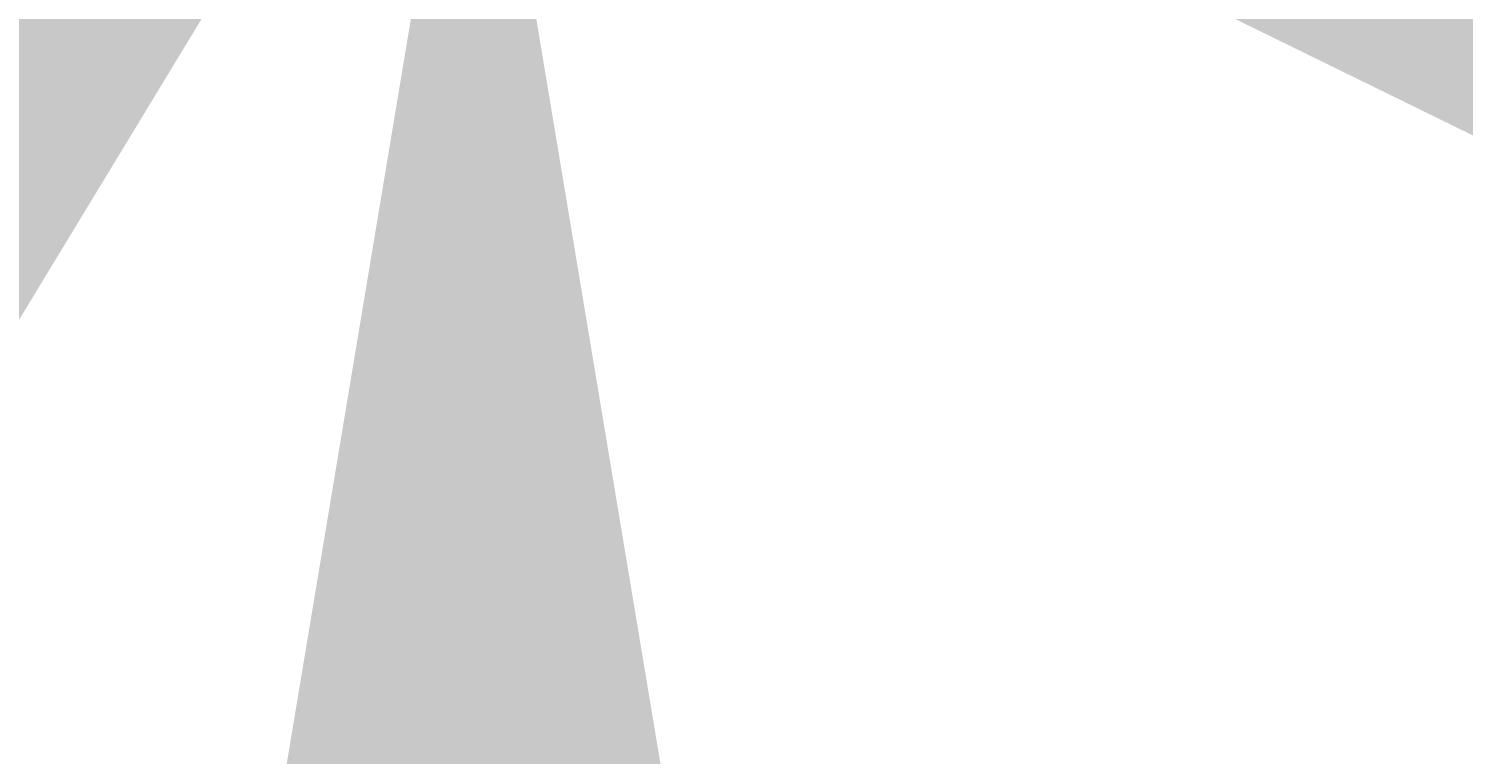
# Model space of a CAD drawing. Units: millimetres. Extents: x -22994 to 29398, y -19990 to 20176.
# Tile 3 of 135: x -2139 to 5745, y -5973 to -1986. Entities that reach past the tile are written whole.
import ezdxf

# ---------------------------------------------------------------- set-up
doc = ezdxf.new("R2010")
doc.units = ezdxf.units.MM
doc.header["$MEASUREMENT"] = 0
doc.layers.add('M-DIMS', color=2, linetype='Continuous', lineweight=18)
doc.styles.get("Standard").update_dxf_attribs({"font": 'arial.ttf'})
doc.dimstyles.get("Standard").update_dxf_attribs({"dimtxt": 0.18, "dimasz": 10000, "dimexe": 0.18, "dimexo": 0.0625, "dimgap": 0.09, "dimtad": 0, "dimtih": 1, "dimtoh": 1, "dimdec": 0, "dimzin": 0, "dimdsep": 46, "dimtxsty": 'Standard', "dimcen": 0.09, "dimadec": 0, "dimazin": 0, "dimtfac": 1, "dimtdec": 0, "dimtofl": 0, "dimtmove": 0, "dimatfit": 3, "dimfxl": 1, "dimtolj": 1, "dimtzin": 0, "dimlwd": 30, "dimarcsym": 0})

# ---------------------------------------------------------------- blocks, each defined once
blk = doc.blocks.new('*D9')
at = {"layer": 'Defpoints', "color": 0, "transparency": 16777216}
for p in [(187.3, 176.4), (306.2, 176.4), (290.9, 10.3)]:
    blk.add_point(p, dxfattribs=at)
at = {"layer": 'M-DIMS', "color": 0, "lineweight": 30, "transparency": 16777216}
for p, q in [((306.2, 10176.4), (306.2, 20176.4)), ((306.2, -9989.7), (306.2, -19989.7))]:
    blk.add_line(p, q, dxfattribs=at)
at = {"layer": 'M-DIMS', "color": 0, "lineweight": -2, "transparency": 16777216}
for p, q in [((187.3, 176.4), (306.4, 176.4)), ((290.9, 10.3), (306.4, 10.3))]:
    blk.add_line(p, q, dxfattribs=at)
at = {"layer": 'M-DIMS', "color": 0, "transparency": 16777216}
for points in [[(-1360.5, 10176.4), (1972.9, 10176.4), (306.2, 176.4)], [(-1360.5, -9989.7), (1972.9, -9989.7), (306.2, 10.3)]]:
    blk.add_solid(points, dxfattribs=at)
at = {"layer": 'M-DIMS', "color": 0, "transparency": 16777216, "insert": (306.2, 93.3), "char_height": 0.18, "attachment_point": 5}
blk.add_mtext('\\A1;166.1', dxfattribs=at)
blk = doc.blocks.new('*D15')
at = {"layer": 'Defpoints', "color": 0, "transparency": 16777216}
for p in [(173.3, 154.8), (173.3, 136.1), (306.2, 136.1)]:
    blk.add_point(p, dxfattribs=at)
at = {"layer": 'M-DIMS', "color": 0, "lineweight": 30, "transparency": 16777216}
for p, q in [((306.2, 10154.8), (306.2, 20154.8)), ((306.2, -9863.9), (306.2, -19863.9))]:
    blk.add_line(p, q, dxfattribs=at)
at = {"layer": 'M-DIMS', "color": 0, "lineweight": -2, "transparency": 16777216}
for p, q in [((173.4, 154.8), (306.4, 154.8)), ((173.4, 136.1), (306.4, 136.1))]:
    blk.add_line(p, q, dxfattribs=at)
at = {"layer": 'M-DIMS', "color": 0, "transparency": 16777216}
for points in [[(-1360.5, 10154.8), (1972.9, 10154.8), (306.2, 154.8)], [(-1360.5, -9863.9), (1972.9, -9863.9), (306.2, 136.1)]]:
    blk.add_solid(points, dxfattribs=at)
at = {"layer": 'M-DIMS', "color": 0, "transparency": 16777216, "insert": (306.2, 145.4), "char_height": 0.18, "attachment_point": 5}
blk.add_mtext('\\A1;18.717', dxfattribs=at)
blk = doc.blocks.new('*D28')
at = {"layer": 'Defpoints', "color": 0, "transparency": 16777216}
for p in [(188.1, 48), (188.1, 31), (306.2, 48)]:
    blk.add_point(p, dxfattribs=at)
at = {"layer": 'M-DIMS', "color": 0, "lineweight": 30, "transparency": 16777216}
for p, q in [((306.2, 10048), (306.2, 20048)), ((306.2, -9969), (306.2, -19969))]:
    blk.add_line(p, q, dxfattribs=at)
at = {"layer": 'M-DIMS', "color": 0, "lineweight": -2, "transparency": 16777216}
for p, q in [((188.2, 48), (306.4, 48)), ((188.2, 31), (306.4, 31))]:
    blk.add_line(p, q, dxfattribs=at)
at = {"layer": 'M-DIMS', "color": 0, "transparency": 16777216}
for points in [[(-1360.5, 10048), (1972.9, 10048), (306.2, 48)], [(-1360.5, -9969), (1972.9, -9969), (306.2, 31)]]:
    blk.add_solid(points, dxfattribs=at)
at = {"layer": 'M-DIMS', "color": 0, "transparency": 16777216, "insert": (306.2, 39.5), "char_height": 0.18, "attachment_point": 5}
blk.add_mtext('\\A1;17.045', dxfattribs=at)
blk = doc.blocks.new('*D32')
at = {"layer": 'Defpoints', "color": 0, "transparency": 16777216}
for p in [(52.4, 113.1), (57.2, 118.6)]:
    blk.add_point(p, dxfattribs=at)
at = {"layer": 'M-DIMS', "color": 0, "lineweight": -2, "transparency": 16777216}
for p, q in [((57.1, 118.6), (57.3, 118.6)), ((57.2, 118.5), (57.2, 118.7))]:
    blk.add_line(p, q, dxfattribs=at)
at = {"layer": 'M-DIMS', "color": 0, "lineweight": 30, "transparency": 16777216}
for p, q in [((-12992.5, -15047), (-6470.1, -7467)), ((-22992.5, -15047), (-12992.5, -15047))]:
    blk.add_line(p, q, dxfattribs=at)
at = {"layer": 'M-DIMS', "color": 0, "transparency": 16777216}
blk.add_solid([(-7733.4, -6379.9), (-5206.7, -8554), (52.4, 113.1)], dxfattribs=at)
at = {"layer": 'M-DIMS', "color": 0, "transparency": 16777216, "insert": (-22993.2, -15047), "char_height": 0.18, "attachment_point": 5}
blk.add_mtext('\\A1;2X R7.284', dxfattribs=at)
blk = doc.blocks.new('*D33')
at = {"layer": 'Defpoints', "color": 0, "transparency": 16777216}
for p in [(229.6, 154.4), (233, 153.4)]:
    blk.add_point(p, dxfattribs=at)
at = {"layer": 'M-DIMS', "color": 0, "lineweight": -2, "transparency": 16777216}
for p, q in [((229.5, 154.4), (229.7, 154.4)), ((229.6, 154.3), (229.6, 154.5))]:
    blk.add_line(p, q, dxfattribs=at)
at = {"layer": 'M-DIMS', "color": 0, "lineweight": 30, "transparency": 16777216}
for p, q in [((19396.3, -5570.8), (9814.7, -2708.7)), ((29396.3, -5570.8), (19396.3, -5570.8))]:
    blk.add_line(p, q, dxfattribs=at)
at = {"layer": 'M-DIMS', "color": 0, "transparency": 16777216}
blk.add_solid([(10291.7, -1111.8), (9337.7, -4305.7), (233, 153.4)], dxfattribs=at)
at = {"layer": 'M-DIMS', "color": 0, "transparency": 16777216, "insert": (29397, -5570.8), "char_height": 0.18, "attachment_point": 5}
blk.add_mtext('\\A1;6X R3.586', dxfattribs=at)

msp = doc.modelspace()

# ---------------------------------------------------------------- dimensions: what is measured, and where the dimension line sits
at = {"layer": 'M-DIMS'}
for base, p1, p2, override, picture, middle in [((306.202, 176.3662), (290.852, 10.2713), (187.2647, 176.3662), {"dimdec": 1, "dimlfac": 1, "dimrnd": 0, "dimzin": 0, "dimdsep": 46, "dimlunit": 2}, '*D9', (306.202, 93.3187)), ((306.202, 136.0713), (173.3459, 154.788), (173.3459, 136.0713), {"dimdec": 3, "dimlfac": 1, "dimrnd": 0, "dimzin": 0, "dimdsep": 46, "dimlunit": 2}, '*D15', (306.202, 145.4297)), ((306.202, 48.0349), (188.1175, 30.9895), (188.1175, 48.0349), {"dimdec": 3, "dimlfac": 1, "dimrnd": 0, "dimzin": 0, "dimdsep": 46, "dimlunit": 2}, '*D28', (306.202, 39.5122))]:
    dim = msp.add_linear_dim(base=base, p1=p1, p2=p2, angle=90, dimstyle='Standard', override=override, dxfattribs=at)
    dim.commit()
    dim.dimension.update_dxf_attribs({"geometry": picture, "text_midpoint": middle})
for center, mpoint, text, picture, middle in [((57.1639, 118.6143), (52.4129, 113.0929), '2X <>', '*D32', (-22993.208, -15047.0314)), ((229.5613, 154.3773), (232.9972, 153.3509), '6X <>', '*D33', (29397.0125, -5570.8378))]:
    dim = msp.add_radius_dim(center=center, mpoint=mpoint, text=text, dimstyle='Standard', override={"dimdec": 3, "dimlfac": 1, "dimrnd": 0, "dimzin": 0, "dimdsep": 46, "dimlunit": 2}, dxfattribs=at)
    dim.commit()
    dim.dimension.update_dxf_attribs({"geometry": picture, "text_midpoint": middle})

doc.saveas('drawing.dxf')
